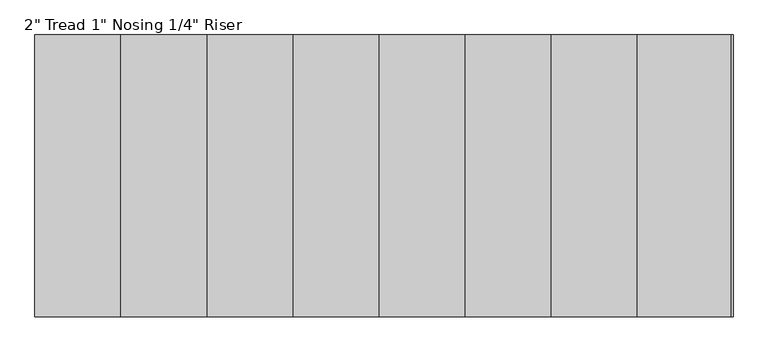
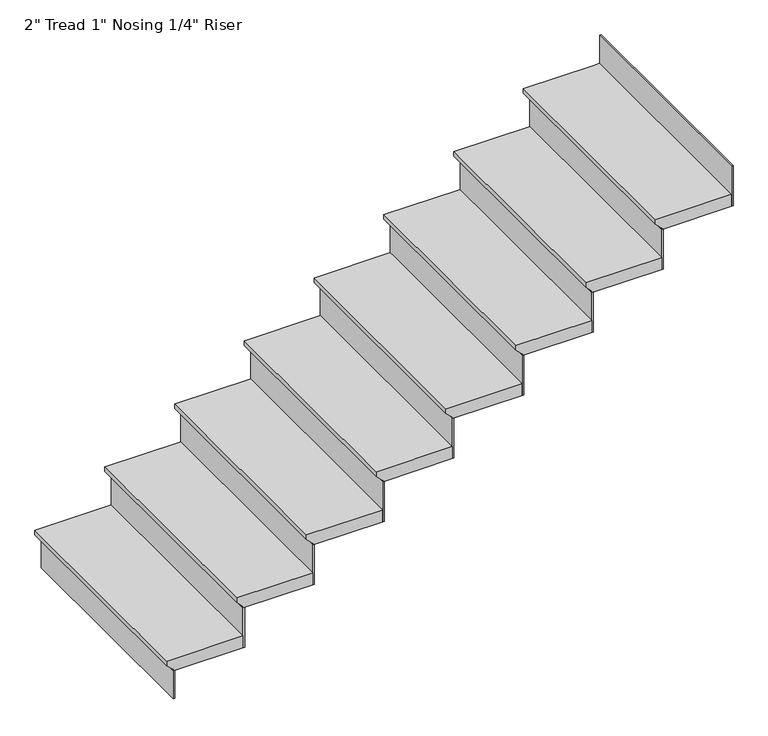
"""IFC4 building model written with IfcOpenShell, lengths in millimetres: stair flight geometry."""

from ifc_helpers import new_model, si_unit, origin, place, context, project, spatial, faceted_brep, source, transform, mapped, element, save


def stair_flight_950fb465(model_context):
    return source(origin(), model_context, "Body", "Brep", [
        faceted_brep([(-12941.4571222, 6754.0964313, 455.0833333), (-12941.4571222, 6754.0964313, 474.1333333), (-12941.4571222, 7668.4964313, 474.1333333), (-12941.4571222, 7668.4964313, 455.0833333), (-12916.0571222, 6754.0964313, 429.6833333), (-12916.0571222, 7668.4964313, 429.6833333), (-12636.6571222, 6754.0964313, 474.1333333), (-12636.6571222, 7668.4964313, 474.1333333), (-12916.0571222, 7668.4964313, 423.3333333), (-12636.6571222, 7668.4964313, 423.3333333), (-12636.6571222, 6754.0964313, 423.3333333), (-12916.0571222, 6754.0964313, 423.3333333)], [[[0, 1, 2, 3]], [[4, 0, 3, 5]], [[2, 1, 6, 7]], [[8, 9, 10, 11]], [[2, 7, 9, 8, 5, 3]], [[8, 11, 4, 5]], [[6, 1, 0, 4, 11, 10]], [[7, 6, 10, 9]]]),
        faceted_brep([(-12916.0571222, 6754.0964313, 423.3333333), (-12916.0571222, 6754.0964313, 304.8), (-12909.7071222, 6754.0964313, 304.8), (-12909.7071222, 6754.0964313, 423.3333333), (-12916.0571222, 7668.4964313, 423.3333333), (-12909.7071222, 7668.4964313, 423.3333333), (-12909.7071222, 7668.4964313, 304.8), (-12916.0571222, 7668.4964313, 304.8)], [[[0, 1, 2, 3]], [[4, 5, 6, 7]], [[1, 0, 4, 7]], [[2, 1, 7, 6]], [[3, 2, 6, 5]], [[0, 3, 5, 4]]]),
        faceted_brep([(-12636.6571222, 6754.0964313, 592.6666667), (-12636.6571222, 6754.0964313, 423.3333333), (-12630.3071222, 6754.0964313, 423.3333333), (-12630.3071222, 6754.0964313, 592.6666667), (-12636.6571222, 7668.4964313, 592.6666667), (-12630.3071222, 7668.4964313, 592.6666667), (-12630.3071222, 7668.4964313, 423.3333333), (-12636.6571222, 7668.4964313, 423.3333333)], [[[0, 1, 2, 3]], [[4, 5, 6, 7]], [[1, 0, 4, 7]], [[2, 1, 7, 6]], [[3, 2, 6, 5]], [[0, 3, 5, 4]]]),
        faceted_brep([(-12662.0571222, 7668.4964313, 643.4666667), (-12662.0571222, 6754.0964313, 643.4666667), (-12357.2571222, 6754.0964313, 643.4666667), (-12357.2571222, 7668.4964313, 643.4666667), (-12636.6571222, 7668.4964313, 592.6666667), (-12357.2571222, 7668.4964313, 592.6666667), (-12357.2571222, 6754.0964313, 592.6666667), (-12636.6571222, 6754.0964313, 592.6666667), (-12636.6571222, 7668.4964313, 599.0166667), (-12662.0571222, 7668.4964313, 624.4166667), (-12636.6571222, 6754.0964313, 599.0166667), (-12662.0571222, 6754.0964313, 624.4166667)], [[[0, 1, 2, 3]], [[4, 5, 6, 7]], [[0, 3, 5, 4, 8, 9]], [[4, 7, 10, 8]], [[2, 1, 11, 10, 7, 6]], [[3, 2, 6, 5]], [[11, 1, 0, 9]], [[10, 11, 9, 8]]]),
        faceted_brep([(-12357.2571222, 6754.0964313, 762.0), (-12357.2571222, 6754.0964313, 592.6666667), (-12350.9071222, 6754.0964313, 592.6666667), (-12350.9071222, 6754.0964313, 762.0), (-12357.2571222, 7668.4964313, 762.0), (-12350.9071222, 7668.4964313, 762.0), (-12350.9071222, 7668.4964313, 592.6666667), (-12357.2571222, 7668.4964313, 592.6666667)], [[[0, 1, 2, 3]], [[4, 5, 6, 7]], [[1, 0, 4, 7]], [[2, 1, 7, 6]], [[3, 2, 6, 5]], [[0, 3, 5, 4]]]),
        faceted_brep([(-12382.6571222, 7668.4964313, 812.8), (-12382.6571222, 6754.0964313, 812.8), (-12077.8571222, 6754.0964313, 812.8), (-12077.8571222, 7668.4964313, 812.8), (-12357.2571222, 7668.4964313, 762.0), (-12077.8571222, 7668.4964313, 762.0), (-12077.8571222, 6754.0964313, 762.0), (-12357.2571222, 6754.0964313, 762.0), (-12357.2571222, 7668.4964313, 768.35), (-12382.6571222, 7668.4964313, 793.75), (-12357.2571222, 6754.0964313, 768.35), (-12382.6571222, 6754.0964313, 793.75)], [[[0, 1, 2, 3]], [[4, 5, 6, 7]], [[0, 3, 5, 4, 8, 9]], [[4, 7, 10, 8]], [[2, 1, 11, 10, 7, 6]], [[3, 2, 6, 5]], [[11, 1, 0, 9]], [[10, 11, 9, 8]]]),
        faceted_brep([(-12077.8571222, 6754.0964313, 931.3333333), (-12077.8571222, 6754.0964313, 762.0), (-12071.5071222, 6754.0964313, 762.0), (-12071.5071222, 6754.0964313, 931.3333333), (-12077.8571222, 7668.4964313, 931.3333333), (-12071.5071222, 7668.4964313, 931.3333333), (-12071.5071222, 7668.4964313, 762.0), (-12077.8571222, 7668.4964313, 762.0)], [[[0, 1, 2, 3]], [[4, 5, 6, 7]], [[1, 0, 4, 7]], [[2, 1, 7, 6]], [[3, 2, 6, 5]], [[0, 3, 5, 4]]]),
        faceted_brep([(-12103.2571222, 7668.4964313, 982.1333333), (-12103.2571222, 6754.0964313, 982.1333333), (-11798.4571222, 6754.0964313, 982.1333333), (-11798.4571222, 7668.4964313, 982.1333333), (-12077.8571222, 7668.4964313, 931.3333333), (-11798.4571222, 7668.4964313, 931.3333333), (-11798.4571222, 6754.0964313, 931.3333333), (-12077.8571222, 6754.0964313, 931.3333333), (-12077.8571222, 7668.4964313, 937.6833333), (-12103.2571222, 7668.4964313, 963.0833333), (-12077.8571222, 6754.0964313, 937.6833333), (-12103.2571222, 6754.0964313, 963.0833333)], [[[0, 1, 2, 3]], [[4, 5, 6, 7]], [[0, 3, 5, 4, 8, 9]], [[4, 7, 10, 8]], [[2, 1, 11, 10, 7, 6]], [[3, 2, 6, 5]], [[11, 1, 0, 9]], [[10, 11, 9, 8]]]),
        faceted_brep([(-11798.4571222, 6754.0964313, 1100.6666667), (-11798.4571222, 6754.0964313, 931.3333333), (-11792.1071222, 6754.0964313, 931.3333333), (-11792.1071222, 6754.0964313, 1100.6666667), (-11798.4571222, 7668.4964313, 1100.6666667), (-11792.1071222, 7668.4964313, 1100.6666667), (-11792.1071222, 7668.4964313, 931.3333333), (-11798.4571222, 7668.4964313, 931.3333333)], [[[0, 1, 2, 3]], [[4, 5, 6, 7]], [[1, 0, 4, 7]], [[2, 1, 7, 6]], [[3, 2, 6, 5]], [[0, 3, 5, 4]]]),
        faceted_brep([(-11823.8571222, 7668.4964313, 1151.4666667), (-11823.8571222, 6754.0964313, 1151.4666667), (-11519.0571222, 6754.0964313, 1151.4666667), (-11519.0571222, 7668.4964313, 1151.4666667), (-11798.4571222, 7668.4964313, 1100.6666667), (-11519.0571222, 7668.4964313, 1100.6666667), (-11519.0571222, 6754.0964313, 1100.6666667), (-11798.4571222, 6754.0964313, 1100.6666667), (-11798.4571222, 7668.4964313, 1107.0166667), (-11823.8571222, 7668.4964313, 1132.4166667), (-11798.4571222, 6754.0964313, 1107.0166667), (-11823.8571222, 6754.0964313, 1132.4166667)], [[[0, 1, 2, 3]], [[4, 5, 6, 7]], [[0, 3, 5, 4, 8, 9]], [[4, 7, 10, 8]], [[2, 1, 11, 10, 7, 6]], [[3, 2, 6, 5]], [[11, 1, 0, 9]], [[10, 11, 9, 8]]]),
        faceted_brep([(-11519.0571222, 6754.0964313, 1270.0), (-11519.0571222, 6754.0964313, 1100.6666667), (-11512.7071222, 6754.0964313, 1100.6666667), (-11512.7071222, 6754.0964313, 1270.0), (-11519.0571222, 7668.4964313, 1270.0), (-11512.7071222, 7668.4964313, 1270.0), (-11512.7071222, 7668.4964313, 1100.6666667), (-11519.0571222, 7668.4964313, 1100.6666667)], [[[0, 1, 2, 3]], [[4, 5, 6, 7]], [[1, 0, 4, 7]], [[2, 1, 7, 6]], [[3, 2, 6, 5]], [[0, 3, 5, 4]]]),
        faceted_brep([(-11544.4571222, 7668.4964313, 1320.8), (-11544.4571222, 6754.0964313, 1320.8), (-11239.6571222, 6754.0964313, 1320.8), (-11239.6571222, 7668.4964313, 1320.8), (-11519.0571222, 7668.4964313, 1270.0), (-11239.6571222, 7668.4964313, 1270.0), (-11239.6571222, 6754.0964313, 1270.0), (-11519.0571222, 6754.0964313, 1270.0), (-11519.0571222, 7668.4964313, 1276.35), (-11544.4571222, 7668.4964313, 1301.75), (-11519.0571222, 6754.0964313, 1276.35), (-11544.4571222, 6754.0964313, 1301.75)], [[[0, 1, 2, 3]], [[4, 5, 6, 7]], [[0, 3, 5, 4, 8, 9]], [[4, 7, 10, 8]], [[2, 1, 11, 10, 7, 6]], [[3, 2, 6, 5]], [[11, 1, 0, 9]], [[10, 11, 9, 8]]]),
        faceted_brep([(-11239.6571222, 6754.0964313, 1439.3333333), (-11239.6571222, 6754.0964313, 1270.0), (-11233.3071222, 6754.0964313, 1270.0), (-11233.3071222, 6754.0964313, 1439.3333333), (-11239.6571222, 7668.4964313, 1439.3333333), (-11233.3071222, 7668.4964313, 1439.3333333), (-11233.3071222, 7668.4964313, 1270.0), (-11239.6571222, 7668.4964313, 1270.0)], [[[0, 1, 2, 3]], [[4, 5, 6, 7]], [[1, 0, 4, 7]], [[2, 1, 7, 6]], [[3, 2, 6, 5]], [[0, 3, 5, 4]]]),
        faceted_brep([(-11265.0571222, 7668.4964313, 1490.1333333), (-11265.0571222, 6754.0964313, 1490.1333333), (-10960.2571222, 6754.0964313, 1490.1333333), (-10960.2571222, 7668.4964313, 1490.1333333), (-11239.6571222, 7668.4964313, 1439.3333333), (-10960.2571222, 7668.4964313, 1439.3333333), (-10960.2571222, 6754.0964313, 1439.3333333), (-11239.6571222, 6754.0964313, 1439.3333333), (-11239.6571222, 7668.4964313, 1445.6833333), (-11265.0571222, 7668.4964313, 1471.0833333), (-11239.6571222, 6754.0964313, 1445.6833333), (-11265.0571222, 6754.0964313, 1471.0833333)], [[[0, 1, 2, 3]], [[4, 5, 6, 7]], [[0, 3, 5, 4, 8, 9]], [[4, 7, 10, 8]], [[2, 1, 11, 10, 7, 6]], [[3, 2, 6, 5]], [[11, 1, 0, 9]], [[10, 11, 9, 8]]]),
        faceted_brep([(-10680.8571222, 6754.0964313, 1778.0), (-10680.8571222, 6754.0964313, 1608.6666667), (-10674.5071222, 6754.0964313, 1608.6666667), (-10674.5071222, 6754.0964313, 1778.0), (-10680.8571222, 7668.4964313, 1778.0), (-10674.5071222, 7668.4964313, 1778.0), (-10674.5071222, 7668.4964313, 1608.6666667), (-10680.8571222, 7668.4964313, 1608.6666667)], [[[0, 1, 2, 3]], [[4, 5, 6, 7]], [[1, 0, 4, 7]], [[2, 1, 7, 6]], [[3, 2, 6, 5]], [[0, 3, 5, 4]]]),
        faceted_brep([(-10960.2571222, 6754.0964313, 1608.6666667), (-10960.2571222, 6754.0964313, 1439.3333333), (-10953.9071222, 6754.0964313, 1439.3333333), (-10953.9071222, 6754.0964313, 1608.6666667), (-10960.2571222, 7668.4964313, 1608.6666667), (-10953.9071222, 7668.4964313, 1608.6666667), (-10953.9071222, 7668.4964313, 1439.3333333), (-10960.2571222, 7668.4964313, 1439.3333333)], [[[0, 1, 2, 3]], [[4, 5, 6, 7]], [[1, 0, 4, 7]], [[2, 1, 7, 6]], [[3, 2, 6, 5]], [[0, 3, 5, 4]]]),
        faceted_brep([(-10680.8571222, 7668.4964313, 1659.4666667), (-10706.2571222, 7668.4964313, 1659.4666667), (-10985.6571222, 7668.4964313, 1659.4666667), (-10985.6571222, 6754.0964313, 1659.4666667), (-10680.8571222, 6754.0964313, 1659.4666667), (-10706.2571222, 7668.4964313, 1608.6666667), (-10680.8571222, 7668.4964313, 1608.6666667), (-10680.8571222, 6754.0964313, 1608.6666667), (-10960.2571222, 6754.0964313, 1608.6666667), (-10960.2571222, 7668.4964313, 1608.6666667), (-10960.2571222, 7668.4964313, 1615.0166667), (-10985.6571222, 7668.4964313, 1640.4166667), (-10960.2571222, 6754.0964313, 1615.0166667), (-10985.6571222, 6754.0964313, 1640.4166667)], [[[0, 1, 2, 3, 4]], [[5, 6, 7, 8, 9]], [[1, 0, 6, 5]], [[2, 1, 5, 9, 10, 11]], [[9, 8, 12, 10]], [[4, 3, 13, 12, 8, 7]], [[0, 4, 7, 6]], [[13, 3, 2, 11]], [[12, 13, 11, 10]]]),
    ])


if __name__ == "__main__":
    model = new_model("IFC4")
    model_context = context("Model", 3, world=origin())
    ifc_project = project(units=[si_unit("LENGTHUNIT", "METRE", prefix="MILLI")], contexts=[model_context])
    site = spatial("IfcSite", under=ifc_project)
    building = spatial("IfcBuilding", under=site)
    placement = place(None, origin())
    stair_flight_shape = stair_flight_950fb465(model_context)
    element("IfcStairFlight", 1, ObjectType="2\" Tread 1\" Nosing 1/4\" Riser", at=placement, inside=building, context=model_context, shape_type="MappedRepresentation", body=[
        mapped(stair_flight_shape, transform((0.0, 0.0, 0.0), x_axis=(1.0, 0.0, 0.0), y_axis=(0.0, 1.0, 0.0), z_axis=(0.0, 0.0, 1.0))),
    ])
    save(model, "model.ifc")
